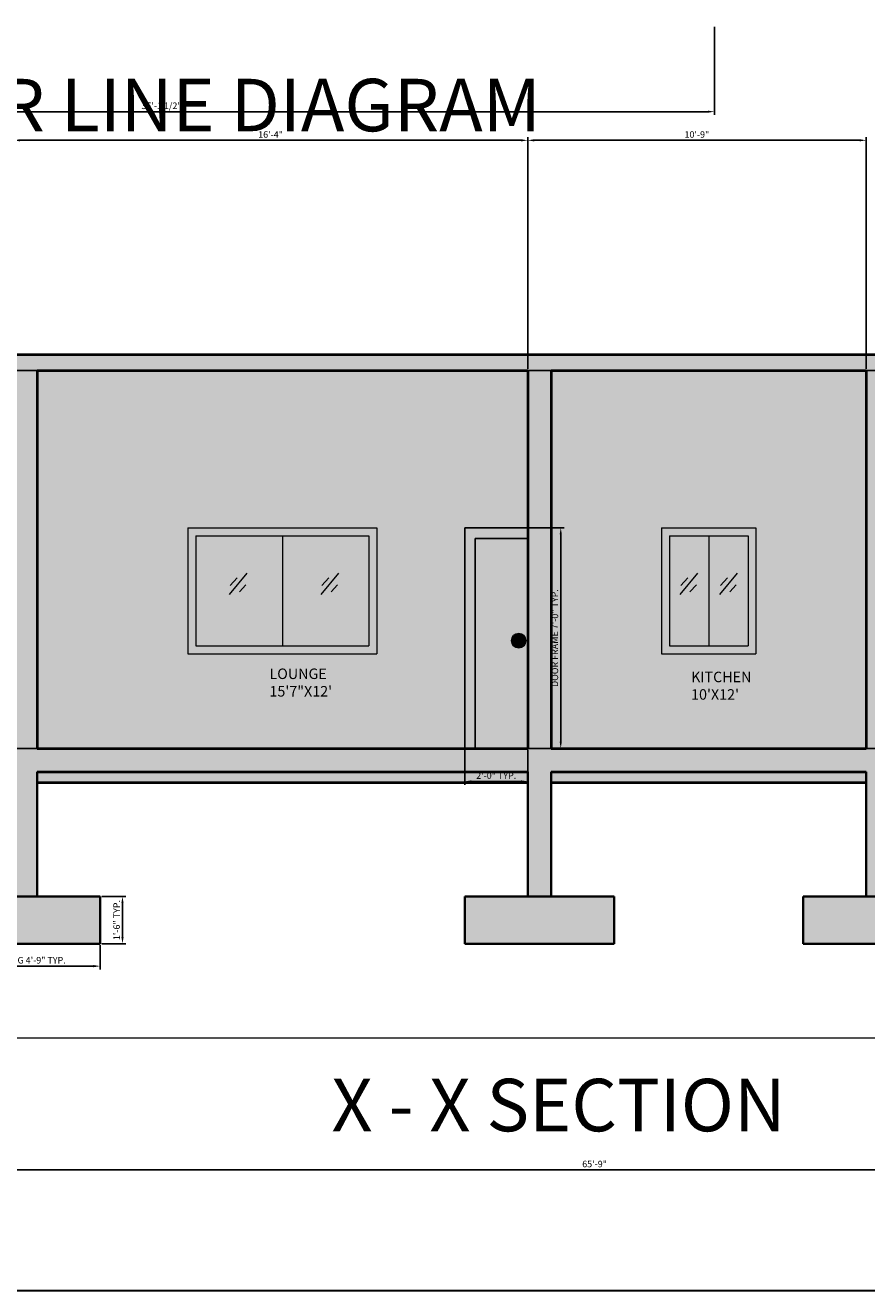
# Model space of a CAD drawing. Units: inches. Extents: x 2163 to 7246, y 928 to 2098.
# Tile 6 of 15: x 2928 to 3249, y 928 to 1411. Entities that reach past the tile are written whole.
import ezdxf

# ---------------------------------------------------------------- set-up
doc = ezdxf.new("R2010")
doc.units = ezdxf.units.IN
for name, color, linetype, lineweight in [('A-ANNO-DIMS', 4, 'Continuous', 18), ('A-ANNO-TITL', 4, 'Continuous', 30), ('A-ANNO-TTLB', 7, 'Continuous', 30), ('A-AREA-IDEN', 7, 'Continuous', 18), ('A-DOOR', 4, 'Continuous', 25), ('A-DOOR-PATT', 35, 'Continuous', 9), ('A-GLAZ', 30, 'Continuous', 20), ('A-SECT', 7, 'Continuous', 40), ('A-SECT-CUT-PATT', 250, 'Continuous', 13), ('S-FNDN', 7, 'Continuous', 35), ('S-FNDN-PATT', 252, 'Continuous', 13)]:
    doc.layers.add(name, color=color, linetype=linetype, lineweight=lineweight)
doc.layers.add('A-GLAZ-PATT', color=141, linetype='Continuous', lineweight=9, true_color=0xadddf7)
doc.layers.add('A-SECT-PATT', color=51, linetype='Continuous', lineweight=9, true_color=0xf8f6b0)
doc.styles.get("Standard").update_dxf_attribs({"font": 'arial.ttf'})
doc.dimstyles.new('ISO-25', dxfattribs={"dimtxt": 2.5, "dimasz": 2.5, "dimexe": 1.25, "dimexo": 0.625, "dimtad": 1, "dimdec": 0, "dimlunit": 3, "dimtxsty": 'Standard', "dimcen": 2.5, "dimadec": 0, "dimazin": 0, "dimtfac": 1, "dimtdec": 0, "dimtmove": 0, "dimatfit": 3, "dimfxl": 1, "dimarcsym": 0})

# ---------------------------------------------------------------- blocks, each defined once
blk = doc.blocks.new('FOOTING-57X18-SECTION')
for p, q in [((24, 18), (0, 18)), ((0, 18), (0, 0)), ((57, 18), (24, 18)), ((57, 0), (57, 18)), ((0, 0), (24, 0)), ((24, 0), (57, 0))]:
    blk.add_line(p, q)
blk = doc.blocks.new('WIN-36X48-FRAME-SECTION')
for p, q in [((0, 48), (36, 48)), ((0, 48), (0, 0)), ((3, 45), (33, 45)), ((3, 45), (3, 3)), ((18, 45), (18, 3)), ((33, 45), (33, 3)), ((36, 48), (36, 0)), ((0, 0), (36, 0)), ((3, 3), (33, 3))]:
    blk.add_line(p, q)
blk = doc.blocks.new('DOOR-FRAME-SECTION')
for p, q in [((0, 84), (0, 0)), ((0, 84), (24, 84)), ((4, 80), (24, 80)), ((4, 80), (4, 0))]:
    blk.add_line(p, q)
blk = doc.blocks.new('GLAZ-REFLECTION-SECTION')
for p, q in [((0, 0), (6.77, 8.07)), ((0.29, 3.36), (2.9, 6.25)), ((3.76, 0.92), (6.2, 3.64))]:
    blk.add_line(p, q)
blk = doc.blocks.new('*D55')
at = {"layer": 'A-ANNO-DIMS', "color": 0, "lineweight": -2, "transparency": 16777216}
for p, q in [((2899.54, 1060.06), (2899.54, 1050.88)), ((2956.54, 1060.06), (2956.54, 1050.88)), ((2902.04, 1052.13), (2954.04, 1052.13))]:
    blk.add_line(p, q, dxfattribs=at)
at = {"layer": 'A-ANNO-DIMS', "color": 0, "transparency": 16777216}
for points in [[(2902.04, 1052.55), (2902.04, 1051.71), (2899.54, 1052.13)], [(2954.04, 1052.55), (2954.04, 1051.71), (2956.54, 1052.13)]]:
    blk.add_solid(points, dxfattribs=at)
at = {"layer": 'Defpoints', "color": 0, "transparency": 16777216}
for p in [(2899.54, 1060.68), (2956.54, 1060.68), (2956.54, 1052.13)]:
    blk.add_point(p, dxfattribs=at)
at = {"layer": 'A-ANNO-DIMS', "color": 0, "transparency": 16777216, "insert": (2928.04, 1054.05), "char_height": 2.5, "attachment_point": 5}
blk.add_mtext('FOOTING 4\'-9" TYP.', dxfattribs=at)
blk = doc.blocks.new('*D56')
at = {"layer": 'A-ANNO-DIMS', "color": 0, "lineweight": -2, "transparency": 16777216}
for p, q in [((2957.17, 1078.68), (2966.34, 1078.68)), ((2965.09, 1063.18), (2965.09, 1076.18)), ((2957.17, 1060.68), (2966.34, 1060.68))]:
    blk.add_line(p, q, dxfattribs=at)
at = {"layer": 'A-ANNO-DIMS', "color": 0, "transparency": 16777216}
for points in [[(2964.68, 1076.18), (2965.51, 1076.18), (2965.09, 1078.68)], [(2964.68, 1063.18), (2965.51, 1063.18), (2965.09, 1060.68)]]:
    blk.add_solid(points, dxfattribs=at)
at = {"layer": 'Defpoints', "color": 0, "transparency": 16777216}
for p in [(2956.54, 1078.68), (2965.09, 1078.68), (2956.54, 1060.68)]:
    blk.add_point(p, dxfattribs=at)
at = {"layer": 'A-ANNO-DIMS', "color": 0, "transparency": 16777216, "insert": (2963.19, 1069.68), "char_height": 2.5, "attachment_point": 5, "rotation": 90}
blk.add_mtext('1\'-6" TYP.', dxfattribs=at)
blk = doc.blocks.new('*D61')
at = {"layer": 'A-ANNO-DIMS', "color": 0, "lineweight": -2, "transparency": 16777216}
for p, q in [((3120.17, 1219.11), (3133.39, 1219.11)), ((3132.14, 1137.61), (3132.14, 1216.61)), ((3120.17, 1135.11), (3133.39, 1135.11))]:
    blk.add_line(p, q, dxfattribs=at)
at = {"layer": 'A-ANNO-DIMS', "color": 0, "transparency": 16777216}
for points in [[(3131.73, 1216.61), (3132.56, 1216.61), (3132.14, 1219.11)], [(3131.73, 1137.61), (3132.56, 1137.61), (3132.14, 1135.11)]]:
    blk.add_solid(points, dxfattribs=at)
at = {"layer": 'Defpoints', "color": 0, "transparency": 16777216}
for p in [(3119.54, 1219.11), (3132.14, 1219.11), (3119.54, 1135.11)]:
    blk.add_point(p, dxfattribs=at)
at = {"layer": 'A-ANNO-DIMS', "color": 0, "transparency": 16777216, "insert": (3130.23, 1177.11), "char_height": 2.5, "attachment_point": 5, "rotation": 90}
blk.add_mtext('DOOR FRAME 7\'-0" TYP.', dxfattribs=at)
blk = doc.blocks.new('*D62')
at = {"layer": 'A-ANNO-DIMS', "color": 0, "lineweight": -2, "transparency": 16777216}
for p, q in [((3095.54, 1134.48), (3095.54, 1121.26)), ((3119.54, 1134.48), (3119.54, 1121.26)), ((3098.04, 1122.51), (3117.04, 1122.51))]:
    blk.add_line(p, q, dxfattribs=at)
at = {"layer": 'A-ANNO-DIMS', "color": 0, "transparency": 16777216}
for points in [[(3098.04, 1122.92), (3098.04, 1122.09), (3095.54, 1122.51)], [(3117.04, 1122.92), (3117.04, 1122.09), (3119.54, 1122.51)]]:
    blk.add_solid(points, dxfattribs=at)
at = {"layer": 'Defpoints', "color": 0, "transparency": 16777216}
for p in [(3095.54, 1135.11), (3119.54, 1135.11), (3119.54, 1122.51)]:
    blk.add_point(p, dxfattribs=at)
at = {"layer": 'A-ANNO-DIMS', "color": 0, "transparency": 16777216, "insert": (3107.54, 1124.41), "char_height": 2.5, "attachment_point": 5}
blk.add_mtext('2\'-0" TYP.', dxfattribs=at)
blk = doc.blocks.new('*D79')
at = {"layer": 'A-ANNO-DIMS', "color": 0, "lineweight": -2, "transparency": 16777216}
for p, q in [((2769.22, 1409.95), (2769.22, 1376.42)), ((3190.72, 1409.95), (3190.72, 1376.42)), ((2771.72, 1377.67), (3188.22, 1377.67))]:
    blk.add_line(p, q, dxfattribs=at)
at = {"layer": 'A-ANNO-DIMS', "color": 0, "transparency": 16777216}
for points in [[(2771.72, 1378.09), (2771.72, 1377.26), (2769.22, 1377.67)], [(3188.22, 1378.09), (3188.22, 1377.26), (3190.72, 1377.67)]]:
    blk.add_solid(points, dxfattribs=at)
at = {"layer": 'Defpoints', "color": 0, "transparency": 16777216}
for p in [(2769.22, 1410.57), (3190.72, 1410.57), (3190.72, 1377.67)]:
    blk.add_point(p, dxfattribs=at)
at = {"layer": 'A-ANNO-DIMS', "color": 0, "transparency": 16777216, "insert": (2979.97, 1379.59), "char_height": 2.5, "attachment_point": 5}
blk.add_mtext('35\'-1 1/2"', dxfattribs=at)
blk = doc.blocks.new('*D100')
at = {"layer": 'A-ANNO-DIMS', "color": 0, "lineweight": -2, "transparency": 16777216}
for p, q in [((2750.54, 1060.06), (2750.54, 973.27)), ((3539.54, 1060.06), (3539.54, 973.27)), ((2753.04, 974.52), (3537.04, 974.52))]:
    blk.add_line(p, q, dxfattribs=at)
at = {"layer": 'A-ANNO-DIMS', "color": 0, "transparency": 16777216}
for points in [[(2753.04, 974.94), (2753.04, 974.11), (2750.54, 974.52)], [(3537.04, 974.94), (3537.04, 974.11), (3539.54, 974.52)]]:
    blk.add_solid(points, dxfattribs=at)
at = {"layer": 'Defpoints', "color": 0, "transparency": 16777216}
for p in [(2750.54, 1060.68), (3539.54, 1060.68), (3539.54, 974.52)]:
    blk.add_point(p, dxfattribs=at)
at = {"layer": 'A-ANNO-DIMS', "color": 0, "transparency": 16777216, "insert": (3145.04, 976.42), "char_height": 2.5, "attachment_point": 5}
blk.add_mtext('65\'-9"', dxfattribs=at)
blk = doc.blocks.new('*D103')
at = {"layer": 'A-ANNO-DIMS', "color": 0, "lineweight": -2, "transparency": 16777216}
for p, q in [((2923.54, 1279.73), (2923.54, 1368.01)), ((2926.04, 1366.76), (3117.04, 1366.76)), ((3119.54, 1279.73), (3119.54, 1368.01))]:
    blk.add_line(p, q, dxfattribs=at)
at = {"layer": 'A-ANNO-DIMS', "color": 0, "transparency": 16777216}
for points in [[(2926.04, 1367.17), (2926.04, 1366.34), (2923.54, 1366.76)], [(3117.04, 1367.17), (3117.04, 1366.34), (3119.54, 1366.76)]]:
    blk.add_solid(points, dxfattribs=at)
at = {"layer": 'Defpoints', "color": 0, "transparency": 16777216}
for p in [(3119.54, 1366.76), (2923.54, 1279.11), (3119.54, 1279.11)]:
    blk.add_point(p, dxfattribs=at)
at = {"layer": 'A-ANNO-DIMS', "color": 0, "transparency": 16777216, "insert": (3021.54, 1368.66), "char_height": 2.5, "attachment_point": 5}
blk.add_mtext('16\'-4"', dxfattribs=at)
blk = doc.blocks.new('*D104')
at = {"layer": 'A-ANNO-DIMS', "color": 0, "lineweight": -2, "transparency": 16777216}
for p, q in [((3119.54, 1279.73), (3119.54, 1368.01)), ((3122.04, 1366.76), (3246.04, 1366.76)), ((3248.54, 1279.73), (3248.54, 1368.01))]:
    blk.add_line(p, q, dxfattribs=at)
at = {"layer": 'A-ANNO-DIMS', "color": 0, "transparency": 16777216}
for points in [[(3122.04, 1367.17), (3122.04, 1366.34), (3119.54, 1366.76)], [(3246.04, 1367.17), (3246.04, 1366.34), (3248.54, 1366.76)]]:
    blk.add_solid(points, dxfattribs=at)
at = {"layer": 'Defpoints', "color": 0, "transparency": 16777216}
for p in [(3248.54, 1366.76), (3119.54, 1279.11), (3248.54, 1279.11)]:
    blk.add_point(p, dxfattribs=at)
at = {"layer": 'A-ANNO-DIMS', "color": 0, "transparency": 16777216, "insert": (3184.04, 1368.66), "char_height": 2.5, "attachment_point": 5}
blk.add_mtext('10\'-9"', dxfattribs=at)
blk = doc.blocks.new('*D107')
at = {"layer": 'A-ANNO-DIMS', "color": 0, "lineweight": -2, "transparency": 16777216}
for p, q in [((3256.92, 1279.11), (2663.63, 1279.11)), ((2664.88, 1137.61), (2664.88, 1276.61)), ((3256.92, 1135.11), (2663.63, 1135.11))]:
    blk.add_line(p, q, dxfattribs=at)
at = {"layer": 'A-ANNO-DIMS', "color": 0, "transparency": 16777216}
for points in [[(2664.46, 1276.61), (2665.3, 1276.61), (2664.88, 1279.11)], [(2664.46, 1137.61), (2665.3, 1137.61), (2664.88, 1135.11)]]:
    blk.add_solid(points, dxfattribs=at)
at = {"layer": 'Defpoints', "color": 0, "transparency": 16777216}
for p in [(2664.88, 1279.11), (3257.54, 1279.11), (3257.54, 1135.11)]:
    blk.add_point(p, dxfattribs=at)
at = {"layer": 'A-ANNO-DIMS', "color": 0, "transparency": 16777216, "insert": (2662.98, 1207.11), "char_height": 2.5, "attachment_point": 5, "rotation": 90}
blk.add_mtext('12\'-0"', dxfattribs=at)

msp = doc.modelspace()

# ---------------------------------------------------------------- hatches: boundary and pattern name
at = {"layer": 'A-DOOR-PATT'}
h = msp.add_hatch(color=256, dxfattribs=at)
h.dxf.hatch_style = 1
h.paths.add_polyline_path([(3350.54, 1219.11), (3350.54, 1215.11), (3370.54, 1215.11), (3370.54, 1135.11), (3374.54, 1135.11), (3374.54, 1219.11)])
h.paths.add_polyline_path([(3119.54, 1215.11), (3119.54, 1219.11), (3095.54, 1219.11), (3095.54, 1135.11), (3099.54, 1135.11), (3099.54, 1215.11)])
h.paths.add_polyline_path([(2923.54, 1215.11), (2923.54, 1219.11), (2899.54, 1219.11), (2899.54, 1135.11), (2903.54, 1135.11), (2903.54, 1215.11)])
h = msp.add_hatch(color=256, dxfattribs=at)
h.dxf.hatch_style = 1
h.paths.add_polyline_path([(2923.54, 1215.11), (2903.54, 1215.11), (2903.54, 1135.11), (2923.54, 1135.11)])
h.paths.add_polyline_path([(2921.06, 1176.14, -1), (2915.61, 1176.14, -1)], flags=16)
h.paths.add_polyline_path([(2920.22, 1176.14, -1), (2916.45, 1176.14, -1)], flags=0)
h.paths.add_polyline_path([(3099.54, 1135.11), (3119.54, 1135.11), (3119.54, 1215.11), (3099.54, 1215.11)])
h.paths.add_polyline_path([(3118.83, 1176.14, -1), (3113.38, 1176.14, -1)], flags=16)
h.paths.add_polyline_path([(3117.99, 1176.14, -1), (3114.22, 1176.14, -1)], flags=0)
h.paths.add_polyline_path([(3370.54, 1215.11), (3350.54, 1215.11), (3350.54, 1135.11), (3370.54, 1135.11)])
h.paths.add_polyline_path([(3356.37, 1176.14, -1), (3350.92, 1176.14, -1)], flags=16)
h.paths.add_polyline_path([(3355.53, 1176.14, -1), (3351.76, 1176.14, -1)], flags=0)
h = msp.add_hatch(color=256, dxfattribs=at)
h.dxf.hatch_style = 1
h.paths.add_polyline_path([(3113.38, 1176.14, 1), (3118.83, 1176.14, 1)])
h.paths.add_polyline_path([(3117.99, 1176.14, 1), (3114.22, 1176.14, 1)], flags=16)
h = msp.add_hatch(color=256, dxfattribs=at)
h.dxf.hatch_style = 1
h.paths.add_polyline_path([(3114.22, 1176.14, 1), (3117.99, 1176.14, 1)])
at = {"layer": 'A-GLAZ-PATT'}
h = msp.add_hatch(color=256, dxfattribs=at)
h.dxf.hatch_style = 1
h.paths.add_polyline_path([(2874.54, 1216.11), (2853.54, 1216.11), (2853.54, 1174.11), (2874.54, 1174.11)])
h.paths.add_polyline_path([(2853.54, 1216.11), (2832.54, 1216.11), (2832.54, 1174.11), (2853.54, 1174.11)])
h.paths.add_polyline_path([(3026.04, 1216.11), (2993.04, 1216.11), (2993.04, 1174.11), (3026.04, 1174.11)])
h.paths.add_polyline_path([(3059.04, 1216.11), (3026.04, 1216.11), (3026.04, 1174.11), (3059.04, 1174.11)])
h.paths.add_polyline_path([(3188.54, 1216.11), (3173.54, 1216.11), (3173.54, 1174.11), (3188.54, 1174.11)])
h.paths.add_polyline_path([(3203.54, 1216.11), (3188.54, 1216.11), (3188.54, 1174.11), (3203.54, 1174.11)])
h.paths.add_polyline_path([(3332.54, 1216.11), (3314.54, 1216.11), (3314.54, 1204.11), (3332.54, 1204.11)])
h.paths.add_polyline_path([(3428.54, 1216.11), (3413.54, 1216.11), (3413.54, 1174.11), (3428.54, 1174.11)])
h.paths.add_polyline_path([(3443.54, 1216.11), (3428.54, 1216.11), (3428.54, 1174.11), (3443.54, 1174.11)])
at = {"layer": 'A-SECT-CUT-PATT'}
h = msp.add_hatch(color=256, dxfattribs=at)
h.dxf.hatch_style = 1
h.paths.add_polyline_path([(2783.54, 1279.11), (2923.54, 1279.11), (2923.54, 1135.11), (2783.54, 1135.11), (2783.54, 1171.11), (2774.54, 1171.11), (2774.54, 1078.68), (2783.54, 1078.68), (2783.54, 1126.11), (2923.54, 1126.11), (2923.54, 1078.68), (2932.54, 1078.68), (2932.54, 1126.11), (3119.54, 1126.11), (3119.54, 1078.68), (3128.54, 1078.68), (3128.54, 1126.11), (3248.54, 1126.11), (3248.54, 1078.68), (3257.54, 1078.68), (3257.54, 1126.11), (3341.54, 1126.11), (3341.54, 1078.68), (3350.54, 1078.68), (3350.54, 1126.11), (3506.54, 1126.11), (3506.54, 1078.68), (3515.54, 1078.68), (3515.54, 1321.11), (3511.54, 1321.11), (3509.54, 1321.11), (3509.54, 1319.11), (3511.54, 1319.11), (3511.54, 1285.11), (2778.54, 1285.11), (2778.54, 1319.11), (2780.54, 1319.11), (2780.54, 1321.11), (2778.54, 1321.11), (2774.54, 1321.11), (2774.54, 1219.11), (2783.54, 1219.11)])
h.paths.add_polyline_path([(2932.54, 1279.11), (3119.54, 1279.11), (3119.54, 1135.11), (2932.54, 1135.11)], flags=16)
h.paths.add_polyline_path([(2990.04, 1219.11), (3062.04, 1219.11), (3062.04, 1171.11), (2990.04, 1171.11)], flags=0)
h.paths.add_polyline_path([(2993.04, 1216.11), (3059.04, 1216.11), (3059.04, 1174.11), (2993.04, 1174.11)], flags=0)
h.paths.add_polyline_path([(3118.83, 1176.14, -1), (3113.38, 1176.14, -1)], flags=0)
h.paths.add_polyline_path([(3117.99, 1176.14, -1), (3114.22, 1176.14, -1)], flags=0)
h.paths.add_polyline_path([(3128.54, 1279.11), (3248.54, 1279.11), (3248.54, 1135.11), (3128.54, 1135.11)], flags=16)
h.paths.add_polyline_path([(3170.54, 1219.11), (3206.54, 1219.11), (3206.54, 1171.11), (3170.54, 1171.11)], flags=0)
h.paths.add_polyline_path([(3173.54, 1216.11), (3203.54, 1216.11), (3203.54, 1174.11), (3173.54, 1174.11)], flags=0)
h.paths.add_polyline_path([(3257.54, 1279.11), (3341.54, 1279.11), (3341.54, 1135.11), (3257.54, 1135.11)], flags=16)
h.paths.add_polyline_path([(3257.54, 1159.11), (3265.54, 1159.11), (3265.54, 1157.11), (3265.04, 1157.11), (3265.04, 1156.11), (3266.54, 1156.11), (3266.54, 1155.11), (3265.04, 1155.11), (3265.04, 1147.11), (3269.54, 1147.11), (3269.54, 1148.11), (3290.04, 1148.11), (3290.04, 1147.11), (3290.54, 1147.11), (3290.54, 1145.11), (3290.04, 1145.11, -0.188679), (3279.54, 1139.66), (3279.54, 1137.11), (3279.54, 1136.11), (3280.54, 1136.11), (3280.54, 1135.11), (3258.54, 1135.11), (3258.54, 1136.11), (3259.54, 1136.11), (3259.54, 1137.11), (3278.54, 1137.11), (3278.54, 1139.59, 0.204728), (3290.04, 1145.11), (3265.54, 1145.11), (3263.54, 1143.11), (3258.04, 1143.11), (3258.04, 1157.11), (3257.54, 1157.11)], flags=0)
h.paths.add_polyline_path([(3311.54, 1219.11), (3335.54, 1219.11), (3335.54, 1201.11), (3311.54, 1201.11)], flags=0)
h.paths.add_polyline_path([(3314.54, 1216.11), (3332.54, 1216.11), (3332.54, 1204.11), (3314.54, 1204.11)], flags=0)
h.paths.add_polyline_path([(3350.54, 1279.11), (3506.54, 1279.11), (3506.54, 1135.11), (3350.54, 1135.11)], flags=16)
h.paths.add_polyline_path([(3356.37, 1176.14, -1), (3350.92, 1176.14, -1)], flags=0)
h.paths.add_polyline_path([(3355.53, 1176.14, -1), (3351.76, 1176.14, -1)], flags=0)
h.paths.add_polyline_path([(3410.54, 1219.11), (3446.54, 1219.11), (3446.54, 1171.11), (3410.54, 1171.11)], flags=0)
h.paths.add_polyline_path([(3413.54, 1216.11), (3443.54, 1216.11), (3443.54, 1174.11), (3413.54, 1174.11)], flags=0)
h = msp.add_hatch(color=256, dxfattribs=at)
h.dxf.hatch_style = 1
h.paths.add_polyline_path([(2783.54, 1216.11), (2783.54, 1219.11), (2774.54, 1219.11), (2774.54, 1216.11)])
h.paths.add_polyline_path([(2774.54, 1174.11), (2774.54, 1171.11), (2783.54, 1171.11), (2783.54, 1174.11)])
h.paths.add_polyline_path([(2877.54, 1171.11), (2877.54, 1219.11), (2829.54, 1219.11), (2829.54, 1171.11)])
h.paths.add_polyline_path([(2832.54, 1174.11), (2832.54, 1216.11), (2874.54, 1216.11), (2874.54, 1174.11)], flags=16)
h.paths.add_polyline_path([(3062.04, 1171.11), (3062.04, 1219.11), (2990.04, 1219.11), (2990.04, 1171.11)])
h.paths.add_polyline_path([(2993.04, 1174.11), (2993.04, 1216.11), (3059.04, 1216.11), (3059.04, 1174.11)], flags=16)
h.paths.add_polyline_path([(3206.54, 1171.11), (3206.54, 1219.11), (3170.54, 1219.11), (3170.54, 1171.11)])
h.paths.add_polyline_path([(3173.54, 1174.11), (3173.54, 1216.11), (3203.54, 1216.11), (3203.54, 1174.11)], flags=16)
h.paths.add_polyline_path([(3335.54, 1201.11), (3335.54, 1219.11), (3311.54, 1219.11), (3311.54, 1201.11)])
h.paths.add_polyline_path([(3314.54, 1204.11), (3314.54, 1216.11), (3332.54, 1216.11), (3332.54, 1204.11)], flags=16)
h.paths.add_polyline_path([(3446.54, 1171.11), (3446.54, 1219.11), (3410.54, 1219.11), (3410.54, 1171.11)])
h.paths.add_polyline_path([(3413.54, 1174.11), (3413.54, 1216.11), (3443.54, 1216.11), (3443.54, 1174.11)], flags=16)
at = {"layer": 'A-SECT-PATT'}
h = msp.add_hatch(color=256, dxfattribs=at)
h.dxf.hatch_style = 1
h.paths.add_polyline_path([(2783.54, 1279.11), (2783.54, 1135.11), (2899.54, 1135.11), (2899.54, 1219.11), (2923.54, 1219.11), (2923.54, 1279.11)])
h.paths.add_polyline_path([(2877.54, 1219.11), (2877.54, 1171.11), (2829.54, 1171.11), (2829.54, 1219.11)], flags=16)
h.paths.add_polyline_path([(2874.54, 1216.11), (2874.54, 1174.11), (2832.54, 1174.11), (2832.54, 1216.11)], flags=0)
h.paths.add_polyline_path([(2932.54, 1279.11), (2932.54, 1135.11), (3095.54, 1135.11), (3095.54, 1219.11), (3119.54, 1219.11), (3119.54, 1279.11)])
h.paths.add_polyline_path([(3062.04, 1219.11), (3062.04, 1171.11), (2990.04, 1171.11), (2990.04, 1219.11)], flags=16)
h.paths.add_polyline_path([(3059.04, 1216.11), (3059.04, 1174.11), (2993.04, 1174.11), (2993.04, 1216.11)], flags=0)
h.paths.add_polyline_path([(3128.54, 1135.11), (3248.54, 1135.11), (3248.54, 1279.11), (3128.54, 1279.11)])
h.paths.add_polyline_path([(3170.54, 1219.11), (3206.54, 1219.11), (3206.54, 1171.11), (3170.54, 1171.11)], flags=16)
h.paths.add_polyline_path([(3173.54, 1216.11), (3203.54, 1216.11), (3203.54, 1174.11), (3173.54, 1174.11)], flags=0)
h.paths.add_polyline_path([(3257.54, 1159.11), (3265.54, 1159.11), (3265.54, 1157.11), (3265.04, 1157.11), (3265.04, 1156.11), (3266.54, 1156.11), (3266.54, 1155.11), (3265.04, 1155.11), (3265.04, 1147.11), (3269.54, 1147.11), (3269.54, 1148.11), (3290.04, 1148.11), (3290.04, 1147.11), (3290.54, 1147.11), (3290.54, 1145.11), (3290.04, 1145.11, -0.188679), (3279.54, 1139.66), (3279.54, 1137.11), (3279.54, 1136.11), (3280.54, 1136.11), (3280.54, 1135.11), (3341.54, 1135.11), (3341.54, 1279.11), (3257.54, 1279.11)])
h.paths.add_polyline_path([(3311.54, 1219.11), (3335.54, 1219.11), (3335.54, 1201.11), (3311.54, 1201.11)], flags=16)
h.paths.add_polyline_path([(3314.54, 1216.11), (3332.54, 1216.11), (3332.54, 1204.11), (3314.54, 1204.11)], flags=0)
h.paths.add_polyline_path([(3350.54, 1279.11), (3350.54, 1219.11), (3374.54, 1219.11), (3374.54, 1135.11), (3506.54, 1135.11), (3506.54, 1279.11)])
h.paths.add_polyline_path([(3446.54, 1219.11), (3446.54, 1171.11), (3410.54, 1171.11), (3410.54, 1219.11)], flags=16)
h.paths.add_polyline_path([(3443.54, 1216.11), (3443.54, 1174.11), (3413.54, 1174.11), (3413.54, 1216.11)], flags=0)
h.paths.add_polyline_path([(2835.76, 1152.2), (2883.7, 1152.2), (2883.7, 1167.12), (2835.76, 1167.12)], flags=24)
h.paths.add_polyline_path([(3019.5, 1152.59), (3045.3, 1152.59), (3045.3, 1167.51), (3019.5, 1167.51)], flags=24)
h.paths.add_polyline_path([(3180.22, 1151.37), (3206.95, 1151.37), (3206.95, 1166.3), (3180.22, 1166.3)], flags=24)
h.paths.add_polyline_path([(3284.73, 1152.43), (3319.02, 1152.43), (3319.02, 1167.36), (3284.73, 1167.36)], flags=24)
h.paths.add_polyline_path([(3421.37, 1151.92), (3452.45, 1151.92), (3452.45, 1166.85), (3421.37, 1166.85)], flags=24)
at = {"layer": 'S-FNDN-PATT'}
h = msp.add_hatch(color=256, dxfattribs=at)
h.dxf.hatch_style = 1
h.paths.add_polyline_path([(2783.54, 1126.11), (2783.54, 1122.11), (2923.54, 1122.11), (2923.54, 1126.11)])
h.paths.add_polyline_path([(2932.54, 1126.11), (2932.54, 1122.11), (3119.54, 1122.11), (3119.54, 1126.11)])
h.paths.add_polyline_path([(3128.54, 1126.11), (3128.54, 1122.11), (3248.54, 1122.11), (3248.54, 1126.11)])
h.paths.add_polyline_path([(3341.54, 1122.11), (3341.54, 1126.11), (3257.54, 1126.11), (3257.54, 1122.11)])
h.paths.add_polyline_path([(3350.54, 1126.11), (3350.54, 1122.11), (3506.54, 1122.11), (3506.54, 1126.11)])
h = msp.add_hatch(color=256, dxfattribs=at)
h.dxf.hatch_style = 1
h.paths.add_polyline_path([(2807.54, 1060.68), (2807.54, 1078.68), (2774.54, 1078.68), (2750.54, 1078.68), (2750.54, 1060.68), (2774.54, 1060.68)])
h.paths.add_polyline_path([(2923.54, 1060.68), (2956.54, 1060.68), (2956.54, 1078.68), (2923.54, 1078.68), (2899.54, 1078.68), (2899.54, 1060.68)])
h.paths.add_polyline_path([(3119.54, 1060.68), (3152.54, 1060.68), (3152.54, 1078.68), (3119.54, 1078.68), (3095.54, 1078.68), (3095.54, 1060.68)])
h.paths.add_polyline_path([(3248.54, 1078.68), (3224.54, 1078.68), (3224.54, 1060.68), (3248.54, 1060.68), (3281.54, 1060.68), (3281.54, 1078.68)])
h.paths.add_polyline_path([(3374.54, 1060.68), (3374.54, 1078.68), (3341.54, 1078.68), (3317.54, 1078.68), (3317.54, 1060.68), (3341.54, 1060.68)])
h.paths.add_polyline_path([(3539.54, 1060.68), (3539.54, 1078.68), (3506.54, 1078.68), (3482.54, 1078.68), (3482.54, 1060.68), (3506.54, 1060.68)])

# ---------------------------------------------------------------- linework, layer by layer
at = {"layer": 'A-ANNO-DIMS'}
msp.add_line((2774.54, 1024.87), (3515.54, 1024.87), dxfattribs=at)
at = {"layer": 'A-ANNO-TTLB'}
msp.add_lwpolyline([(2162.62, 2098.21), (3633.38, 2098.21), (3633.38, 928.48), (2162.62, 928.48)], close=True, dxfattribs=at)
at = {"layer": 'A-DOOR'}
for radius in [2.72, 1.89]:
    msp.add_circle((3116.11, 1176.14), radius, dxfattribs=at)
at = {"layer": 'A-GLAZ'}
for p, q in [((2990.04, 1219.11), (3062.04, 1219.11)), ((2990.04, 1219.11), (2990.04, 1171.11)), ((2993.04, 1216.11), (3059.04, 1216.11)), ((2993.04, 1216.11), (2993.04, 1174.11)), ((3026.04, 1216.11), (3026.04, 1174.11)), ((3059.04, 1216.11), (3059.04, 1174.11)), ((3062.04, 1219.11), (3062.04, 1171.11)), ((2993.04, 1174.11), (3059.04, 1174.11)), ((2990.04, 1171.11), (3062.04, 1171.11))]:
    msp.add_line(p, q, dxfattribs=at)
at = {"layer": 'A-SECT'}
for p, q in [((2778.54, 1285.11), (3511.54, 1285.11)), ((2932.54, 1279.11), (2932.54, 1135.11)), ((2932.54, 1279.11), (3119.54, 1279.11)), ((3119.54, 1279.11), (3119.54, 1135.11)), ((3128.54, 1279.11), (3128.54, 1135.11)), ((3128.54, 1279.11), (3248.54, 1279.11)), ((3248.54, 1279.11), (3248.54, 1135.11)), ((2932.54, 1135.11), (3119.54, 1135.11)), ((3128.54, 1135.11), (3248.54, 1135.11)), ((2932.54, 1126.11), (3119.54, 1126.11)), ((3128.54, 1126.11), (3248.54, 1126.11)), ((2932.54, 1122.11), (3119.54, 1122.11)), ((3128.54, 1122.11), (3248.54, 1122.11))]:
    msp.add_line(p, q, dxfattribs=at)
at = {"layer": 'S-FNDN'}
for p, q in [((2932.54, 1126.11), (2932.54, 1078.68)), ((3119.54, 1126.11), (3119.54, 1078.68)), ((3128.54, 1126.11), (3128.54, 1078.68)), ((3248.54, 1126.11), (3248.54, 1078.68))]:
    msp.add_line(p, q, dxfattribs=at)

# ---------------------------------------------------------------- block references
at = {"layer": 'A-DOOR'}
msp.add_blockref('DOOR-FRAME-SECTION', (3095.54, 1135.11), dxfattribs=at)
at = {"layer": 'A-GLAZ'}
for name, p in [('WIN-36X48-FRAME-SECTION', (3170.54, 1171.11)), ('GLAZ-REFLECTION-SECTION', (3005.9, 1193.76)), ('GLAZ-REFLECTION-SECTION', (3040.82, 1193.76)), ('GLAZ-REFLECTION-SECTION', (3177.65, 1193.76)), ('GLAZ-REFLECTION-SECTION', (3192.78, 1193.76))]:
    msp.add_blockref(name, p, dxfattribs=at)
at = {"layer": 'S-FNDN'}
for p in [(2899.54, 1060.68), (3095.54, 1060.68), (3224.54, 1060.68)]:
    msp.add_blockref('FOOTING-57X18-SECTION', p, dxfattribs=at)

# ---------------------------------------------------------------- texts
at = {"layer": 'A-ANNO-TITL', "char_height": 20, "attachment_point": 1}
for s, width, insert in [('CENTER LINE DIAGRAM', 571.2399, (2832.54, 1390.19)), ('X - X SECTION', 559.3338, (3044.77, 1009.2))]:
    msp.add_mtext_dynamic_manual_height_columns(s, width=width, gutter_width=12.5, heights=[0], dxfattribs=dict(at, insert=insert))
at = {"layer": 'A-AREA-IDEN', "char_height": 4, "attachment_point": 1}
for s, width, insert in [('LOUNGE\\P15\'7"X12\'', 87.766, (3021.11, 1165.52)), ("KITCHEN\\P10'X12'", 58.4074, (3181.83, 1164.31))]:
    msp.add_mtext_dynamic_manual_height_columns(s, width=width, gutter_width=12.5, heights=[0], dxfattribs=dict(at, insert=insert))

# ---------------------------------------------------------------- dimensions: what is measured, and where the dimension line sits
at = {"layer": 'A-ANNO-DIMS'}
for base, p1, p2, picture, middle in [((3190.72, 1377.67), (2769.22, 1410.57), (3190.72, 1410.57), '*D79', (2979.97, 1379.59)), ((3119.54, 1366.76), (2923.54, 1279.11), (3119.54, 1279.11), '*D103', (3021.54, 1368.66)), ((3248.54, 1366.76), (3119.54, 1279.11), (3248.54, 1279.11), '*D104', (3184.04, 1368.66)), ((3539.54, 974.52), (2750.54, 1060.68), (3539.54, 1060.68), '*D100', (3145.04, 976.42))]:
    dim = msp.add_linear_dim(base=base, p1=p1, p2=p2, dimstyle='ISO-25', override={"dimdec": 1, "dimlfac": 1, "dimrnd": 0, "dimzin": 1, "dimdsep": 46, "dimlunit": 4, "dimfrac": 2}, dxfattribs=at)
    dim.commit()
    dim.dimension.update_dxf_attribs({"geometry": picture, "text_midpoint": middle})
dim = msp.add_linear_dim(base=(2664.88, 1279.11), p1=(3257.54, 1135.11), p2=(3257.54, 1279.11), angle=90, dimstyle='ISO-25', override={"dimdec": 1, "dimlfac": 1, "dimrnd": 0, "dimzin": 1, "dimdsep": 46, "dimlunit": 4, "dimfrac": 2}, dxfattribs=at)
dim.commit()
dim.dimension.update_dxf_attribs({"geometry": '*D107', "text_midpoint": (2662.98, 1207.11)})
for base, p1, p2, text, picture, middle in [((3132.14, 1219.11), (3119.54, 1135.11), (3119.54, 1219.11), 'DOOR FRAME <> TYP.', '*D61', (3130.23, 1177.11)), ((2965.09, 1078.68), (2956.54, 1060.68), (2956.54, 1078.68), '<> TYP.', '*D56', (2963.19, 1069.68))]:
    dim = msp.add_linear_dim(base=base, p1=p1, p2=p2, angle=90, text=text, dimstyle='ISO-25', override={"dimdec": 1, "dimlfac": 1, "dimrnd": 0, "dimzin": 1, "dimdsep": 46, "dimlunit": 4, "dimfrac": 2}, dxfattribs=at)
    dim.commit()
    dim.dimension.update_dxf_attribs({"geometry": picture, "text_midpoint": middle})
for base, p1, p2, text, picture, middle in [((3119.54, 1122.51), (3095.54, 1135.11), (3119.54, 1135.11), '<> TYP.', '*D62', (3107.54, 1124.41)), ((2956.54, 1052.13), (2899.54, 1060.68), (2956.54, 1060.68), 'FOOTING <> TYP.', '*D55', (2928.04, 1054.05))]:
    dim = msp.add_linear_dim(base=base, p1=p1, p2=p2, text=text, dimstyle='ISO-25', override={"dimdec": 1, "dimlfac": 1, "dimrnd": 0, "dimzin": 1, "dimdsep": 46, "dimlunit": 4, "dimfrac": 2}, dxfattribs=at)
    dim.commit()
    dim.dimension.update_dxf_attribs({"geometry": picture, "text_midpoint": middle})

doc.saveas('drawing.dxf')
